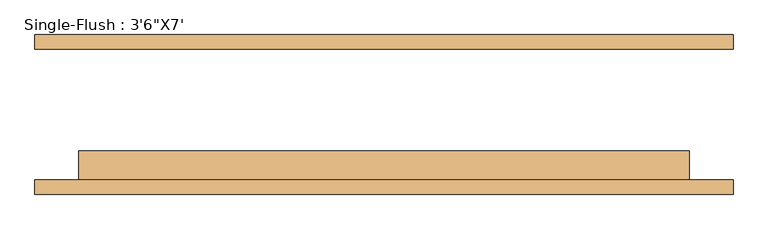
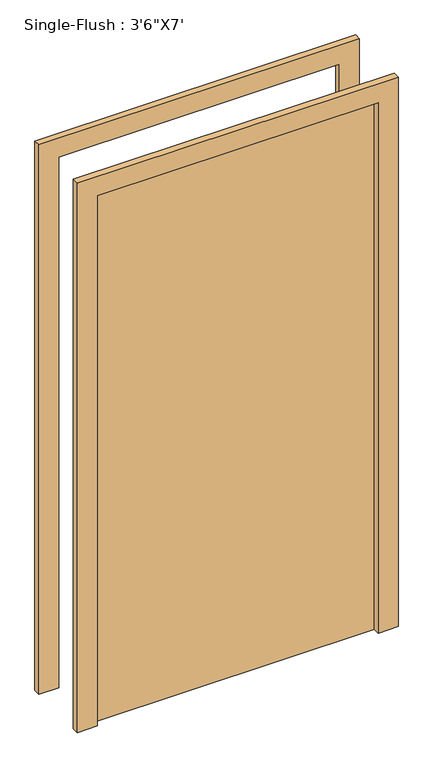
"""IFC4 building model written with IfcOpenShell, lengths in millimetres: door geometry."""

from ifc_helpers import new_model, si_unit, frame, origin, origin_with_axes, place, context, project, spatial, polyline, outline, extrude, source, transform, mapped, element, save


def door_0848dd25(model_context):
    return source(origin(), model_context, "Body", "SweptSolid", [
        extrude(outline(polyline([(2209.8, -609.6), (0.0, -609.6), (0.0, -533.4), (2133.6, -533.4), (2133.6, 533.4), (0.0, 533.4), (0.0, 609.6), (2209.8, 609.6), (2209.8, -609.6)])), frame((0.0, -139.7, 0.0), z_axis=(0.0, 1.0, 0.0), x_axis=(0.0, 0.0, 1.0)), (0.0, 0.0, 1.0), 25.4),
        extrude(outline(polyline([(2209.8, 609.6), (2209.8, -609.6), (0.0, -609.6), (0.0, -533.4), (2133.6, -533.4), (2133.6, 533.4), (0.0, 533.4), (0.0, 609.6), (2209.8, 609.6)])), frame((0.0, 114.3, 0.0), z_axis=(0.0, 1.0, 0.0), x_axis=(0.0, 0.0, 1.0)), (0.0, 0.0, 1.0), 25.4),
        extrude(outline(polyline([(533.4, -63.5), (533.4, -114.3), (-533.4, -114.3), (-533.4, -63.5), (533.4, -63.5)])), origin_with_axes(), (0.0, 0.0, 1.0), 2133.6),
    ])


if __name__ == "__main__":
    model = new_model("IFC4")
    model_context = context("Model", 3, world=origin())
    ifc_project = project(units=[si_unit("LENGTHUNIT", "METRE", prefix="MILLI")], contexts=[model_context])
    site = spatial("IfcSite", under=ifc_project)
    building = spatial("IfcBuilding", under=site)
    placement = place(None, origin())
    door_shape = door_0848dd25(model_context)
    element("IfcDoor", 1, ObjectType="Single-Flush : 3'6\"X7'", at=placement, inside=building, context=model_context, shape_type="MappedRepresentation", body=[
        mapped(door_shape, transform((0.0, 0.0, 0.0), x_axis=(1.0, 0.0, 0.0), y_axis=(0.0, 1.0, 0.0), z_axis=(0.0, 0.0, 1.0))),
    ])
    save(model, "model.ifc")

# Revit data of these elements
# Type "Single-Flush : 3'6\"X7'"
#   Type Mark = "8"
#   Construction Type Id = "MDOOR"
#   Assembly Code = "C1020"
#   Analytic Construction = "Metal"
#   Thickness = 0' - 2"
#   Heat Transfer Coefficient (U) = 0.651978 BTU/(h·ft²·°F)
#   Height = 7' - 0"
#   Trim Projection Ext = 0' - 1"
#   Trim Projection Int = 0' - 1"
#   Trim Width = 0' - 3"
#   Width = 3' - 6"
#   Define Thermal Properties by = 1
#   Door Material = Door - Panel
#   Frame Material = Door - Frame
#   Visual Light Transmittance = 0
#   Solar Heat Gain Coefficient = 0
#   Function = (empty or 0)
#   Wall Closure = (empty or 0)
# Element 1 (IfcDoor, "Single-Flush : 3'6\"X7'")
#   Materials on its faces: "Door - Frame", "Door - Panel"
# Materials
#   "Door - Panel": class "Wood", colour RGB 210 159 95, transparency 0, Cost = 0
#   "Door - Frame": colour RGB 118 70 51, transparency 0, Cost = 0
